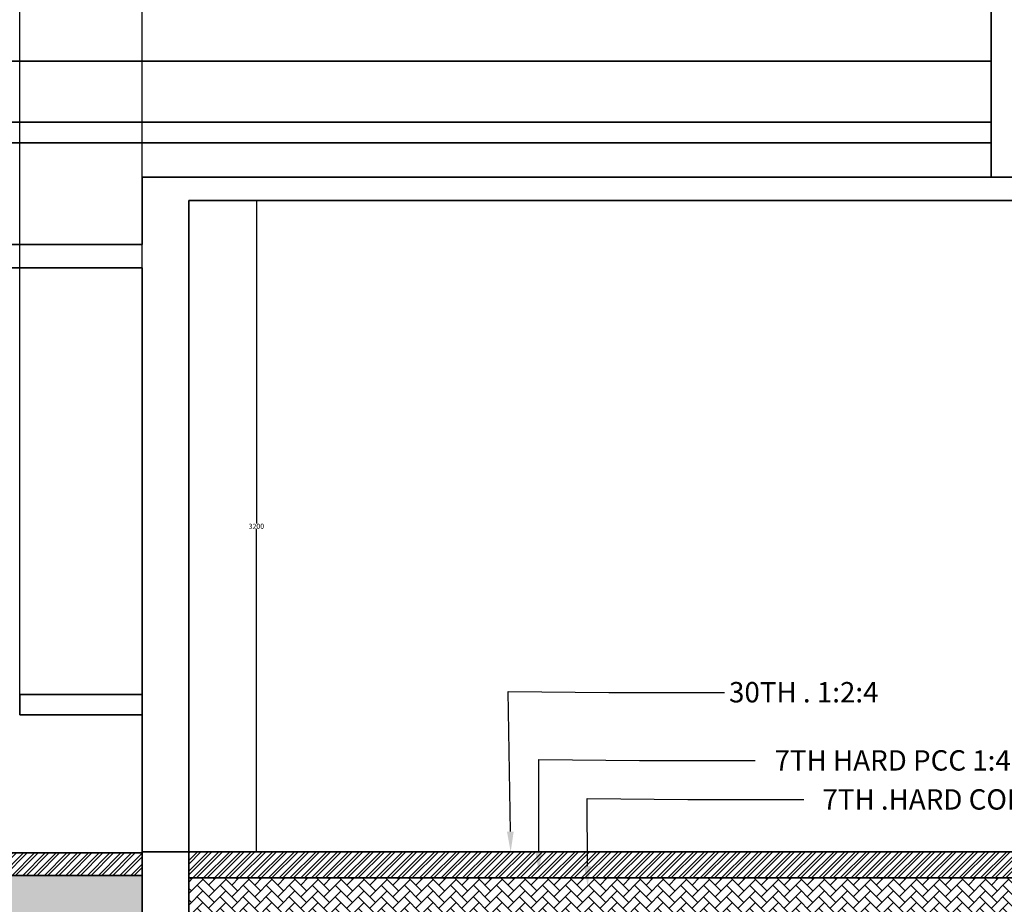
# Model space of a CAD drawing. Units: millimetres. Extents: x 1944 to 29915, y -10550 to 5909.
# Tile 12 of 24: x 11743 to 16582, y -6203 to -1857. Entities that reach past the tile are written whole.
import ezdxf
from ezdxf import colors
from ezdxf.entities.mleader import LeaderData, LeaderLine
from ezdxf.math import Vec2, Vec3

# ---------------------------------------------------------------- set-up
doc = ezdxf.new("R2010")
doc.units = ezdxf.units.MM
doc.header["$MEASUREMENT"] = 0
for name, color, linetype, lineweight in [('A-ANNO-DIMS', 2, 'Continuous', 18), ('A-ANNO-TEXT', 7, 'Continuous', 25), ('A-FLOR-PATT', 252, 'Continuous', 13), ('A-SECT', 7, 'Continuous', 35)]:
    doc.layers.add(name, color=color, linetype=linetype, lineweight=lineweight)
doc.styles.get("Standard").update_dxf_attribs({"font": 'arial.ttf'})
doc.dimstyles.get("Standard").update_dxf_attribs({"dimtxt": 25, "dimasz": 0.18, "dimexe": 0.18, "dimexo": 0.0625, "dimgap": 0.09, "dimtad": 0, "dimtih": 1, "dimtoh": 1, "dimdec": 0, "dimzin": 0, "dimdsep": 46, "dimtxsty": 'Standard', "dimcen": 0.09, "dimadec": 0, "dimazin": 0, "dimtfac": 1, "dimtdec": 0, "dimtofl": 0, "dimtmove": 0, "dimatfit": 3, "dimfxl": 1, "dimtolj": 1, "dimtzin": 0, "dimarcsym": 0})

# ---------------------------------------------------------------- blocks, each defined once
blk = doc.blocks.new('*D24')
at = {"layer": 'A-ANNO-DIMS', "color": 0, "lineweight": -2, "transparency": 16777216}
for p, q in [((12574, -2745.8), (12906.1, -2745.8)), ((12905.9, -2745.9), (12905.9, -4332.9)), ((12905.9, -5945.6), (12905.9, -4358.6)), ((12574, -5945.8), (12906.1, -5945.8))]:
    blk.add_line(p, q, dxfattribs=at)
at = {"layer": 'A-ANNO-DIMS', "color": 0, "transparency": 16777216}
for points in [[(12905.9, -2745.9), (12905.9, -2745.9), (12905.9, -2745.8)], [(12905.9, -5945.6), (12905.9, -5945.6), (12905.9, -5945.8)]]:
    blk.add_solid(points, dxfattribs=at)
at = {"layer": 'Defpoints', "color": 0, "transparency": 16777216}
for p in [(12574, -2745.8), (12574, -5945.8), (12905.9, -5945.8)]:
    blk.add_point(p, dxfattribs=at)
at = {"layer": 'A-ANNO-DIMS', "color": 0, "transparency": 16777216, "insert": (12905.9, -4345.8), "char_height": 25, "attachment_point": 5}
blk.add_mtext('\\A1;3200', dxfattribs=at)
blk = doc.blocks.new('*D93')
at = {"layer": 'A-ANNO-DIMS', "color": 0, "lineweight": -2, "transparency": 16777216}
for p, q in [((11744, -5171.4), (11744, -395.6)), ((11744.2, -395.8), (12016.2, -395.8)), ((12343.8, -395.8), (12071.7, -395.8)), ((12344, -5171.4), (12344, -395.6))]:
    blk.add_line(p, q, dxfattribs=at)
at = {"layer": 'A-ANNO-DIMS', "color": 0, "transparency": 16777216}
for points in [[(11744.2, -395.7), (11744.2, -395.8), (11744, -395.8)], [(12343.8, -395.7), (12343.8, -395.8), (12344, -395.8)]]:
    blk.add_solid(points, dxfattribs=at)
at = {"layer": 'Defpoints', "color": 0, "transparency": 16777216}
for p in [(12344, -395.8), (11744, -5171.5), (12344, -5171.5)]:
    blk.add_point(p, dxfattribs=at)
at = {"layer": 'A-ANNO-DIMS', "color": 0, "transparency": 16777216, "insert": (12044, -395.8), "char_height": 25, "attachment_point": 5}
blk.add_mtext('\\A1;600', dxfattribs=at)

msp = doc.modelspace()

# ---------------------------------------------------------------- hatches: boundary and pattern name
at = {"layer": 'A-FLOR-PATT'}
h = msp.add_hatch(dxfattribs=at)
h.set_pattern_fill('ANSI32', color=256, scale=100)
h.paths.add_polyline_path([(12343.981, -5950.967), (11265.739, -5950.967), (11169.087, -6053.056), (11445.739, -6061.05), (12343.981, -6061.05)])
h = msp.add_hatch(dxfattribs=at)
h.set_pattern_fill('ANSI32', color=256, scale=100)
h.paths.add_polyline_path([(16747.828, -5945.752), (12573.981, -5945.752), (12573.981, -6073.852), (16747.828, -6073.852)])
h = msp.add_hatch(dxfattribs=at)
h.set_pattern_fill('AR-HBONE', color=256, scale=10)
h.paths.add_polyline_path([(12343.981, -6305.752), (12343.981, -6061.05), (11445.739, -6061.05), (11445.739, -6850.967), (11265.739, -6850.967), (10496.11, -6850.967), (10496.11, -6990.545), (6648.315, -6990.545), (6648.315, -7135.877), (12343.981, -7135.877)])
h = msp.add_hatch(dxfattribs=at)
h.set_pattern_fill('AR-HBONE', color=256, scale=10)
h.paths.add_polyline_path([(12573.981, -6073.852), (12573.981, -6305.752), (16747.828, -6305.752), (16747.828, -6073.852)])

# ---------------------------------------------------------------- linework, layer by layer
at = {"layer": 'A-SECT'}
for p, q in [((16516.552, -2630.752), (16516.552, -1730.752)), ((9672.957, -2060.967), (16516.552, -2060.967)), ((9672.957, -2360.967), (16516.552, -2360.967)), ((9695.572, -2460.967), (16516.552, -2460.967)), ((12343.981, -2630.752), (25389.297, -2630.752)), ((12343.981, -2630.752), (12343.981, -2960.967)), ((6418.315, -2960.967), (12343.981, -2960.967)), ((6648.315, -3075.967), (12343.981, -3075.967)), ((12343.981, -5950.967), (12343.981, -3075.967)), ((11743.981, -5271.512), (11743.981, -5171.512)), ((11743.981, -5171.512), (12343.981, -5171.512)), ((12343.981, -5271.512), (11743.981, -5271.512)), ((12343.981, -5950.967), (11265.739, -5950.967)), ((11445.739, -6061.05), (12343.981, -6061.05)), ((12573.981, -6073.852), (16747.828, -6073.852))]:
    msp.add_line(p, q, dxfattribs=at)
for points in [[(12573.981, -2745.752), (16747.828, -2745.752), (16747.828, -5945.752), (12573.981, -5945.752)], [(12343.981, -5945.752), (12573.981, -5945.752), (12573.981, -6305.752), (12343.981, -6305.752)]]:
    msp.add_lwpolyline(points, close=True, dxfattribs=at)

# ---------------------------------------------------------------- dimensions: what is measured, and where the dimension line sits
at = {"layer": 'A-ANNO-DIMS'}
dim = msp.add_linear_dim(base=(12343.981, -395.752), p1=(11743.981, -5171.512), p2=(12343.981, -5171.512), dimstyle='Standard', override={"dimdec": 0, "dimlfac": 1, "dimrnd": 0, "dimzin": 0, "dimdsep": 46, "dimlunit": 2}, dxfattribs=at)
dim.commit()
dim.dimension.update_dxf_attribs({"geometry": '*D93', "text_midpoint": (12043.981, -395.752)})
dim = msp.add_linear_dim(base=(12905.887, -5945.752), p1=(12573.981, -2745.752), p2=(12573.981, -5945.752), angle=90, dimstyle='Standard', override={"dimclrd": 0, "dimclre": 0, "dimclrt": 0}, dxfattribs=at)
dim.commit()
dim.dimension.update_dxf_attribs({"geometry": '*D24', "text_midpoint": (12905.887, -4345.752)})

# ---------------------------------------------------------------- leaders
at = {"layer": 'A-ANNO-TEXT'}
ml = msp.add_multileader_mtext('Standard', dxfattribs=at)
ml.set_content('30TH . 1:2:4', color=256)
ml.set_leader_properties()
ml.build(insert=Vec2(0, 0))
ml.multileader.update_dxf_attribs({"dogleg_length": 568.936, "arrow_head_size": 100})
ctx = ml.context
ctx.base_point, ctx.char_height, ctx.arrow_head_size, ctx.landing_gap_size, ctx.plane_origin = Vec3(15207.031, -5161.907), 100, 100, 0.09, Vec3(14638.095, -5161.907)
ctx.text_align_type = 2
notes = []
notes.append((ctx, [(0, (1, 1, 0), (14638.095, -5161.907), (1, 0), 568.936, [(0, [(14155.715, -5945.752), (14142.71, -5157.054)], 0, [])])]))
ctx.mtext.insert, ctx.mtext.alignment, ctx.mtext.flow_direction = Vec3(15963.26, -5111.021), 3, 5
ml = msp.add_multileader_mtext('Standard', dxfattribs=at)
ml.set_content('7TH HARD PCC 1:4:8', color=256)
ml.set_leader_properties()
ml.build(insert=Vec2(0, 0))
ml.multileader.update_dxf_attribs({"dogleg_length": 568.936, "arrow_head_size": 100})
ctx = ml.context
ctx.base_point, ctx.char_height, ctx.arrow_head_size, ctx.landing_gap_size, ctx.plane_origin = Vec3(15357.883, -5496.91), 100, 100, 0.09, Vec3(14788.948, -5496.91)
ctx.text_align_type = 2
notes.append((ctx, [(0, (1, 1, 0), (14788.948, -5496.91), (1, 0), 568.936, [(0, [(14293.563, -6045.171), (14293.563, -5492.056)], 0, [])])]))
ctx.mtext.insert, ctx.mtext.alignment, ctx.mtext.flow_direction = Vec3(16727.073, -5446.057), 3, 5
ml = msp.add_multileader_mtext('Standard', dxfattribs=at)
ml.set_content('7TH .HARD CORE', color=256)
ml.set_leader_properties()
ml.build(insert=Vec2(0, 0))
ml.multileader.update_dxf_attribs({"dogleg_length": 568.936, "arrow_head_size": 100})
ctx = ml.context
ctx.base_point, ctx.char_height, ctx.arrow_head_size, ctx.landing_gap_size, ctx.plane_origin = Vec3(15595.87, -5688.802), 100, 100, 0.09, Vec3(15026.935, -5688.802)
ctx.text_align_type = 2
notes.append((ctx, [(0, (1, 1, 0), (15026.935, -5688.802), (1, 0), 568.936, [(0, [(14533.534, -6115.34), (14531.55, -5683.948)], 0, [])])]))
ctx.mtext.insert, ctx.mtext.alignment, ctx.mtext.flow_direction = Vec3(16761.649, -5637.949), 3, 5
for ctx, leaders in notes:
    for number, flags, end, landing, length, lines in leaders:
        leader = LeaderData()
        leader.index, (leader.has_last_leader_line, leader.has_dogleg_vector, leader.attachment_direction) = number, flags
        leader.last_leader_point, leader.dogleg_vector, leader.dogleg_length = Vec3(end), Vec3(landing), length
        for number, points, colour, breaks in lines:
            line = LeaderLine()
            line.index, line.vertices, line.color, line.breaks = number, Vec3.list(points), colors.encode_raw_color(colour), breaks
            leader.lines.append(line)
        ctx.leaders.append(leader)

doc.saveas('drawing.dxf')
